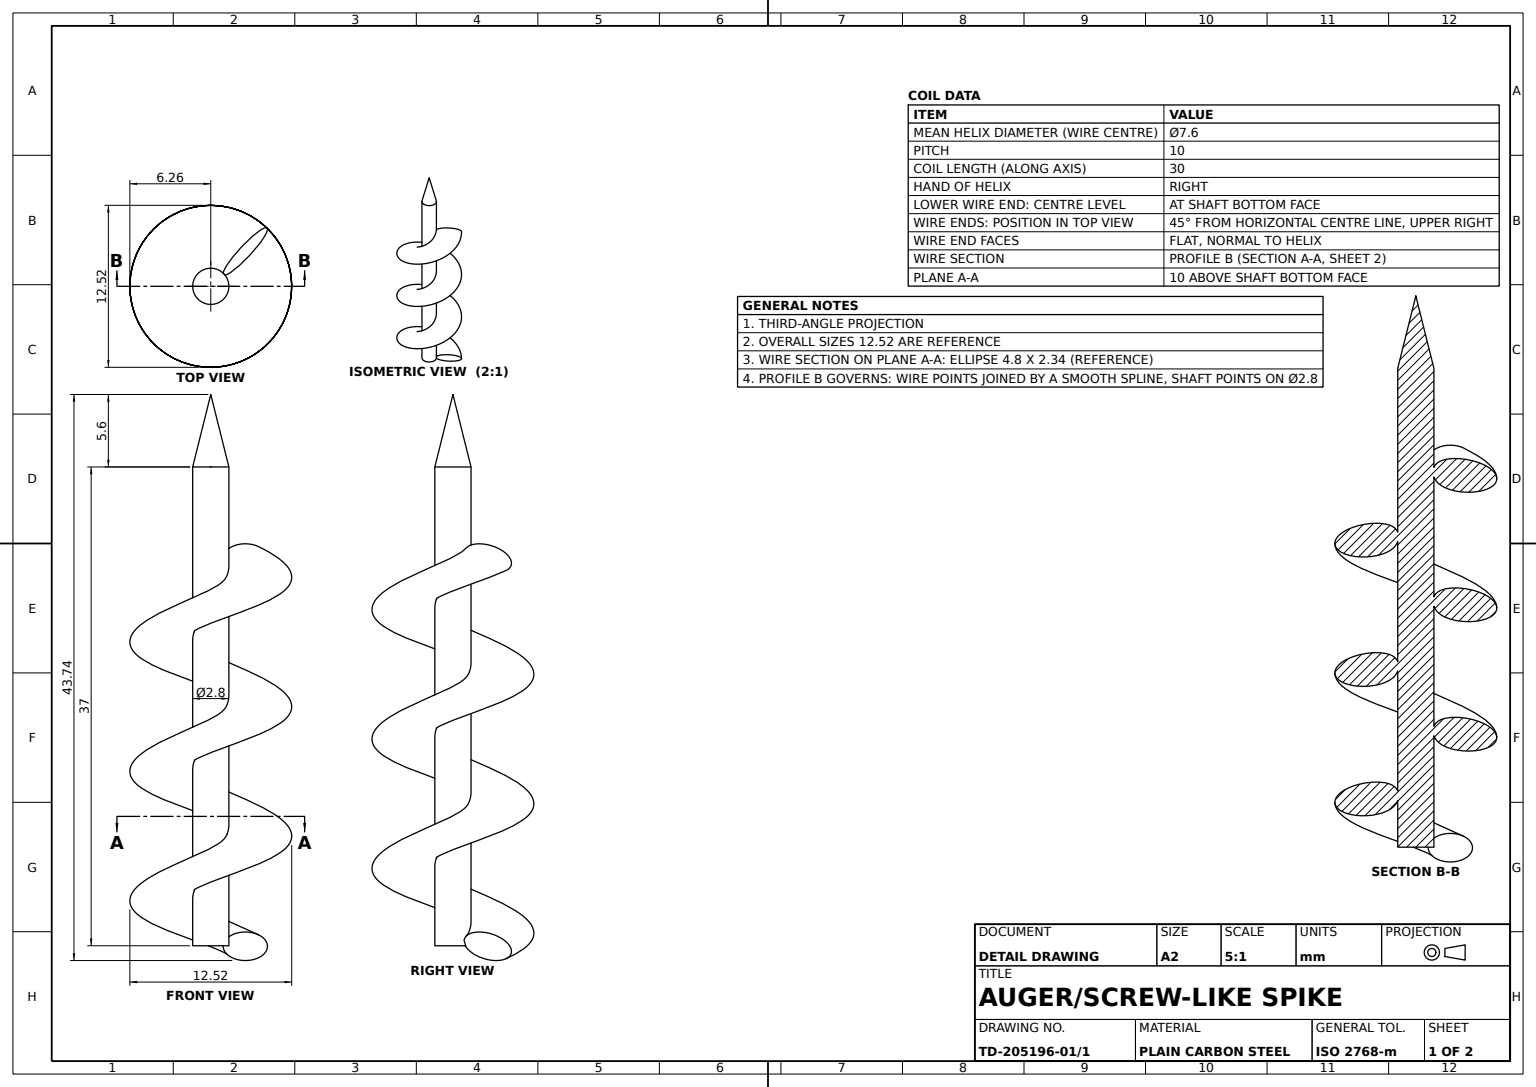
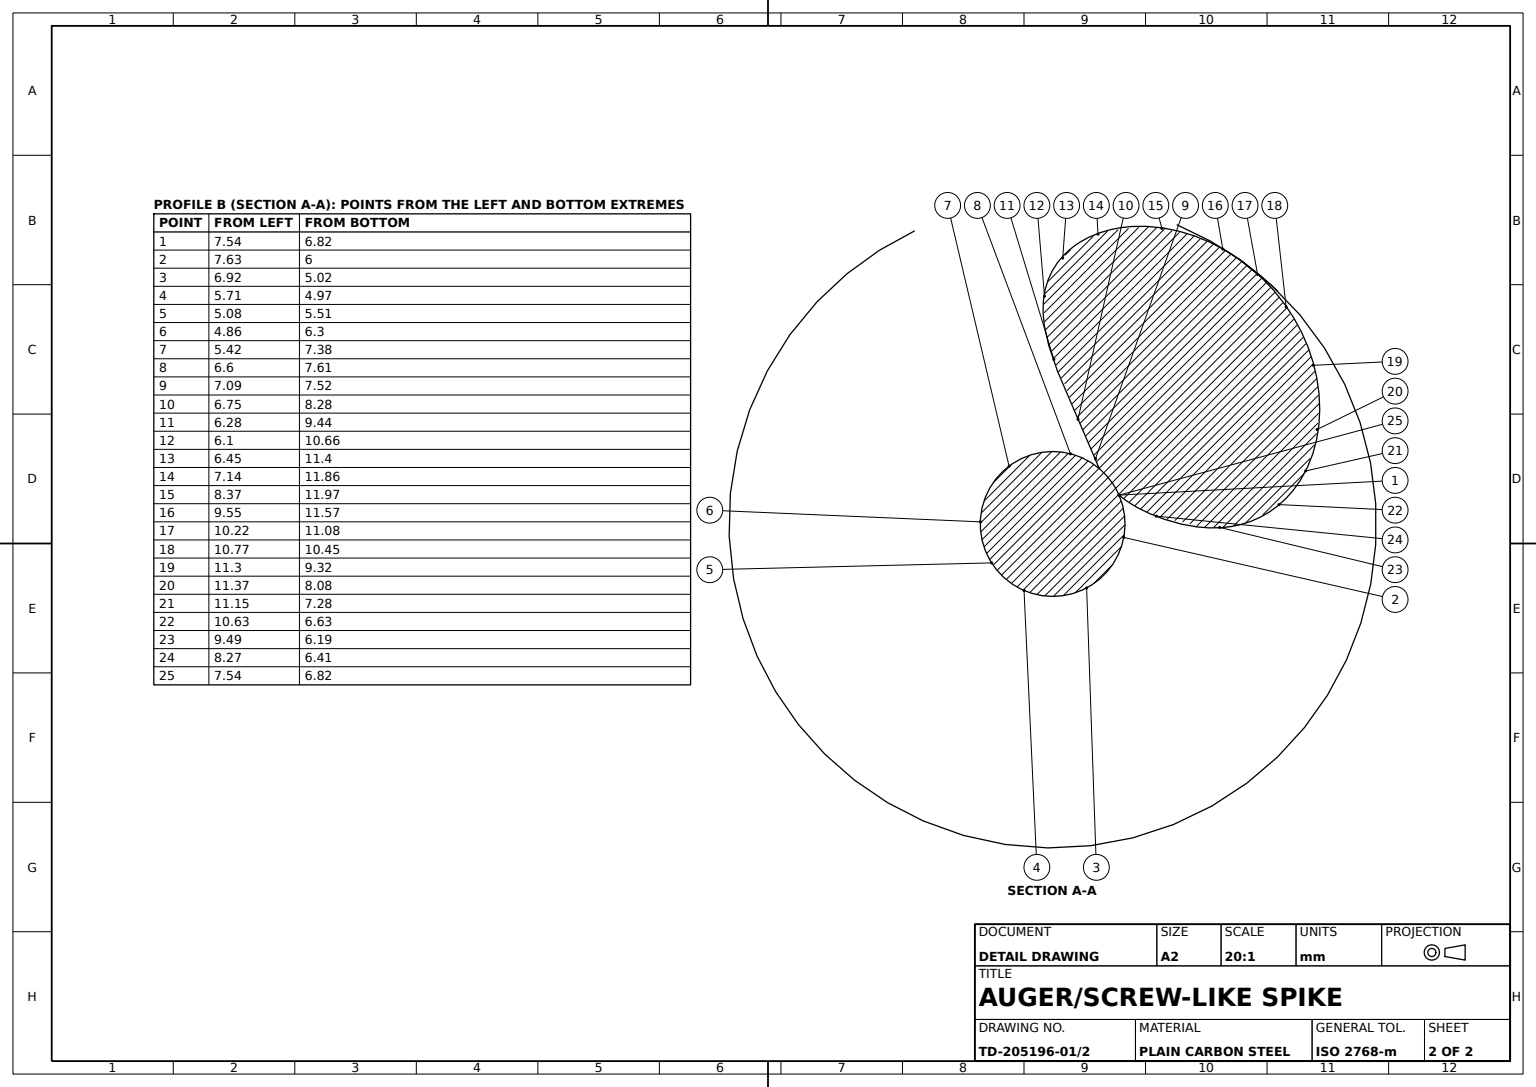
from build123d import *
from build123d.topology import SkipClean

# Parameters (mm, degrees)
SHAFT_SKETCH_R             = 1.4
SHAFT_37MM_DEPTH           = 37
SHAFT_END_CUT_SKETCH_R     = 1.4
SHAFT_END_CUT_10MM_DEPTH   = 10
SHAFT_START                = 10
SHAFT_EXTENSION_SKETCH_R   = 1.4
SHAFT_EXTENSION_10MM_DEPTH = 10
COIL_WIRE_PITCH            = 10
COIL_WIRE_HEIGHT           = 30
COIL_WIRE_RADIUS           = 3.8
COIL_WIRE_START_ANGLE      = 135
COIL_WIRE_PROFILE_RX       = 2.477948864
COIL_WIRE_PROFILE_RY       = 1.169649495


with BuildPart() as part:
    # Shaft Sketch → Shaft 37mm (new body)
    with BuildSketch(Plane(origin=(0, 0, 0), x_dir=(1, 0, 0), z_dir=(0, 1, 0))):
        with Locations(Location((0, 0, 0), (0, 0, 270))):
            Circle(SHAFT_SKETCH_R)
    extrude(amount=SHAFT_37MM_DEPTH)

    # Tip Cone Profile → Conical Tip (revolve)
    with BuildSketch(Plane.XY, mode=Mode.PRIVATE) as conical_tip_sk:
        Polygon((0, 37), (0, 42.6), (1.4, 37), align=None)
    revolve(conical_tip_sk.sketch.rotate(Axis((0, 37, 0), (0, 1, 0)), 90), axis=Axis((0, 37, 0), (0, 1, 0)))

    # Shaft End Cut Sketch → Shaft End Cut 10mm (cut)
    with BuildSketch(Plane.XZ):
        with Locations(Location((0, 0, 0), (0, 0, 270))):
            Circle(SHAFT_END_CUT_SKETCH_R)
    extrude(amount=-SHAFT_END_CUT_10MM_DEPTH, mode=Mode.SUBTRACT)

    # Shaft Extension Sketch → Shaft Extension 10mm (add)
    with BuildSketch(Plane.XZ.offset(-10).offset(SHAFT_START)):
        with Locations(Location((0, 0, 0), (0, 0, 270))):
            Circle(SHAFT_EXTENSION_SKETCH_R)
    extrude(amount=-SHAFT_EXTENSION_10MM_DEPTH)

    # Coil Wire: sweep along a helix
    with SkipClean():  # the faces are left unmerged after this step: merging them gives an invalid solid
        with BuildLine() as coil_wire_path:
            add(Helix(COIL_WIRE_PITCH, COIL_WIRE_HEIGHT, COIL_WIRE_RADIUS, center=(0, 0, 0), direction=(0, 1, 0), mode=Mode.PRIVATE).rotate(Axis((0, 0, 0), (0, 1, 0)), COIL_WIRE_START_ANGLE))
        # Coil Wire Profile → Coil Wire (sweep)
        with BuildSketch(Plane(origin=(2.687005769, 30, -2.687005769), x_dir=(-0.5611613384925322, 0.3323833612114232, 0.758036445938496), z_dir=(-0.652212194480449, 0.3863140001890473, -0.6522121944803959))):
            with Locations(Location((-0.009480676, -0.041804133), (0, 0, -14.409252287))):
                Ellipse(COIL_WIRE_PROFILE_RX, COIL_WIRE_PROFILE_RY)
        sweep(path=coil_wire_path.line, is_frenet=True)


solid = part.part
